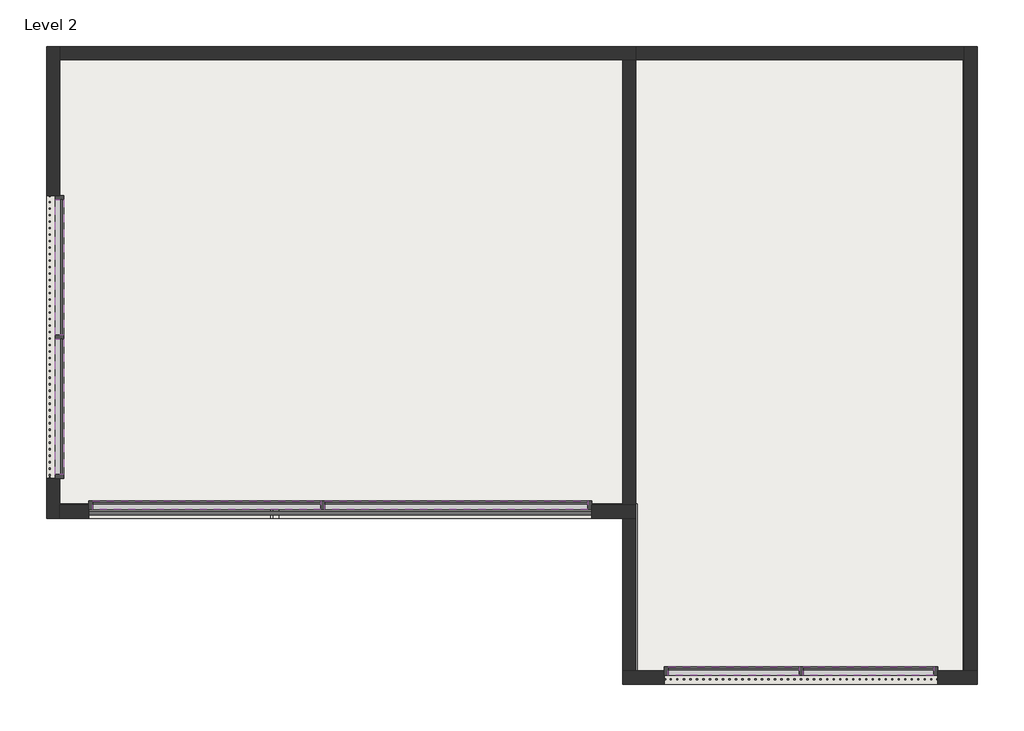
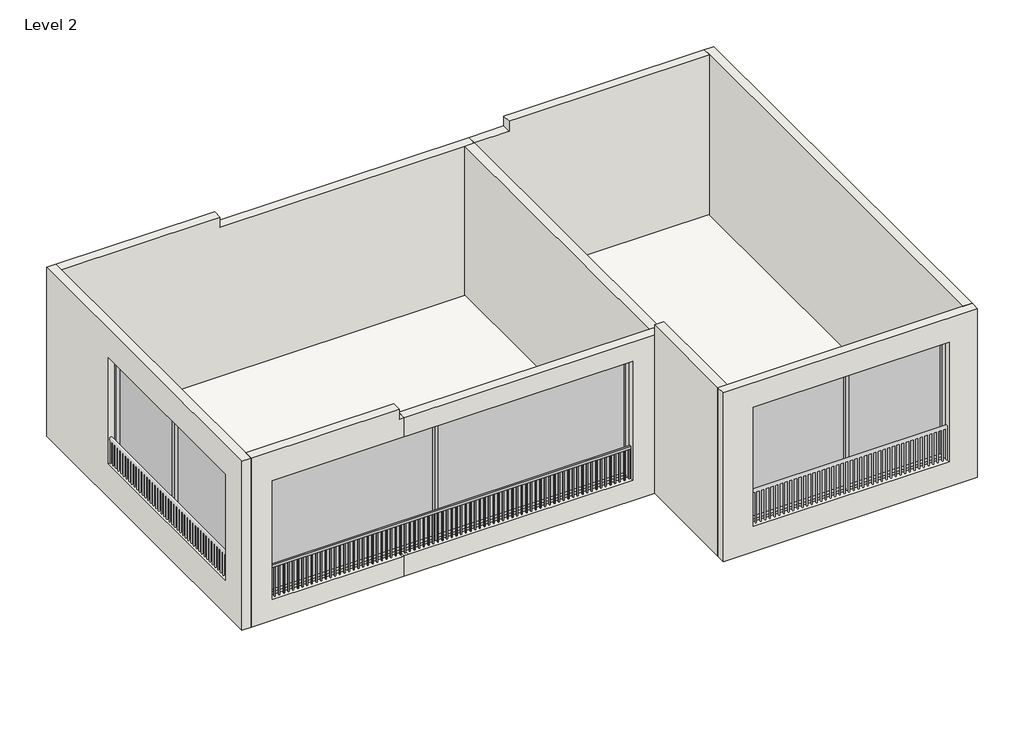
# One storey, part 1 of 2: 21 members, 9 walls, 6 plates, 1 railing, 1 roof.
"""IFC4 building model written with IfcOpenShell, lengths in millimetres."""

from ifc_helpers import new_model, si_unit, frame, origin, place, context, project, spatial, polyline, outline, extrude, faceted_brep, transform, mapped, element, save
from components import member_923d5781, member_d84c53df, member_a78380a5, member_2b402daf, member_c8ecc271, member_8f4b05ff, member_f0fea5a5, member_ee409385, system_panel_glazed_54db570c, system_panel_glazed_4346f86e, system_panel_glazed_ffba6474, system_panel_glazed_48ffcee9

model = new_model("IFC4")

# Units and contexts
model_context = context("Model", 3, world=origin())
ifc_project = project(units=[si_unit("LENGTHUNIT", "METRE", prefix="MILLI")], contexts=[model_context])

# Site, building, storey
site = spatial("IfcSite", under=ifc_project)
building = spatial("IfcBuilding", under=site)
storey = spatial("IfcBuildingStorey", under=building, Name="Level 2", Elevation=3657.6)

# Members
placement = place(None, origin())
member_shape = member_923d5781(model_context)
element("IfcMember", 1, ObjectType="Rectangular Mullion : 2.5\" x 5\" rectangular", at=placement, inside=storey, context=model_context, shape_type="MappedRepresentation", body=[
    mapped(member_shape, transform((-11752.6161748, -214.9874156, 4128.3774754), x_axis=(1.0, 0.0, 0.0), y_axis=(0.0, -1.0, 0.0), z_axis=(0.0, 0.0, -1.0))),
])
element("IfcMember", 2, ObjectType="Rectangular Mullion : 2.5\" x 5\" rectangular", at=placement, inside=storey, context=model_context, shape_type="MappedRepresentation", body=[
    mapped(member_shape, transform((-4288.9796605, -2805.7874156, 4241.0241774), x_axis=(1.0, 0.0, 0.0), y_axis=(0.0, -1.0, 0.0), z_axis=(0.0, 0.0, -1.0))),
])
member_2_shape = member_d84c53df(model_context)
element("IfcMember", 3, ObjectType="Rectangular Mullion : 2.5\" x 5\" rectangular", at=placement, inside=storey, context=model_context, shape_type="MappedRepresentation", body=[
    mapped(member_2_shape, transform((-7616.7372956, -214.9874156, 6871.5774754), x_axis=(0.0, 0.0, 1.0), y_axis=(0.0, -1.0, 0.0), z_axis=(1.0, 0.0, 0.0))),
])
element("IfcMember", 4, ObjectType="Rectangular Mullion : 2.5\" x 5\" rectangular", at=placement, inside=storey, context=model_context, shape_type="MappedRepresentation", body=[
    mapped(member_2_shape, transform((-11720.8661748, -214.9874156, 4128.3774754), x_axis=(0.0, 0.0, -1.0), y_axis=(0.0, -1.0, 0.0), z_axis=(-1.0, 0.0, 0.0))),
])
member_3_shape = member_a78380a5(model_context)
element("IfcMember", 5, ObjectType="Rectangular Mullion : 2.5\" x 5\" rectangular", at=placement, inside=storey, context=model_context, shape_type="MappedRepresentation", body=[
    mapped(member_3_shape, transform((-7553.2372956, -214.9874156, 4128.3774754), x_axis=(1.0, 0.0, 0.0), y_axis=(0.0, -1.0, 0.0), z_axis=(0.0, 0.0, -1.0))),
])
element("IfcMember", 6, ObjectType="Rectangular Mullion : 2.5\" x 5\" rectangular", at=placement, inside=storey, context=model_context, shape_type="MappedRepresentation", body=[
    mapped(member_3_shape, transform((-2155.3796605, -2805.7874156, 4241.0241774), x_axis=(1.0, 0.0, 0.0), y_axis=(0.0, -1.0, 0.0), z_axis=(0.0, 0.0, -1.0))),
])
member_4_shape = member_2b402daf(model_context)
element("IfcMember", 7, ObjectType="Rectangular Mullion : 2.5\" x 5\" rectangular", at=placement, inside=storey, context=model_context, shape_type="MappedRepresentation", body=[
    mapped(member_4_shape, transform((-11784.3661748, -214.9874156, 6871.5774754), x_axis=(0.0, 0.0, 1.0), y_axis=(0.0, -1.0, 0.0), z_axis=(1.0, 0.0, 0.0))),
])
element("IfcMember", 8, ObjectType="Rectangular Mullion : 2.5\" x 5\" rectangular", at=placement, inside=storey, context=model_context, shape_type="MappedRepresentation", body=[
    mapped(member_4_shape, transform((-15346.7161748, -214.9874156, 4128.3774754), x_axis=(0.0, 0.0, -1.0), y_axis=(0.0, -1.0, 0.0), z_axis=(-1.0, 0.0, 0.0))),
])
element("IfcMember", 9, ObjectType="Rectangular Mullion : 2.5\" x 5\" rectangular", at=placement, inside=storey, context=model_context, shape_type="MappedRepresentation", body=[
    mapped(member_3_shape, transform((-15410.2161748, -214.9874156, 6871.5774754), x_axis=(-1.0, 0.0, 0.0), y_axis=(0.0, -1.0, 0.0), z_axis=(0.0, 0.0, 1.0))),
])
element("IfcMember", 10, ObjectType="Rectangular Mullion : 2.5\" x 5\" rectangular", at=placement, inside=storey, context=model_context, shape_type="MappedRepresentation", body=[
    mapped(member_3_shape, transform((-6422.5796605, -2805.7874156, 6984.2241774), x_axis=(-1.0, 0.0, 0.0), y_axis=(0.0, -1.0, 0.0), z_axis=(0.0, 0.0, 1.0))),
])
member_5_shape = member_c8ecc271(model_context)
element("IfcMember", 11, ObjectType="Rectangular Mullion : 2.5\" x 5\" rectangular", at=placement, inside=storey, context=model_context, shape_type="MappedRepresentation", body=[
    mapped(member_5_shape, transform((-4320.7296605, -2805.7874156, 6984.2241774), x_axis=(0.0, 0.0, 1.0), y_axis=(0.0, -1.0, 0.0), z_axis=(1.0, 0.0, 0.0))),
])
element("IfcMember", 12, ObjectType="Rectangular Mullion : 2.5\" x 5\" rectangular", at=placement, inside=storey, context=model_context, shape_type="MappedRepresentation", body=[
    mapped(member_5_shape, transform((-2218.8796605, -2805.7874156, 6984.2241774), x_axis=(0.0, 0.0, 1.0), y_axis=(0.0, -1.0, 0.0), z_axis=(1.0, 0.0, 0.0))),
])
element("IfcMember", 13, ObjectType="Rectangular Mullion : 2.5\" x 5\" rectangular", at=placement, inside=storey, context=model_context, shape_type="MappedRepresentation", body=[
    mapped(member_5_shape, transform((-4257.2296605, -2805.7874156, 4241.0241774), x_axis=(0.0, 0.0, -1.0), y_axis=(0.0, -1.0, 0.0), z_axis=(-1.0, 0.0, 0.0))),
])
element("IfcMember", 14, ObjectType="Rectangular Mullion : 2.5\" x 5\" rectangular", at=placement, inside=storey, context=model_context, shape_type="MappedRepresentation", body=[
    mapped(member_5_shape, transform((-6359.0796605, -2805.7874156, 4241.0241774), x_axis=(0.0, 0.0, -1.0), y_axis=(0.0, -1.0, 0.0), z_axis=(-1.0, 0.0, 0.0))),
])
member_6_shape = member_8f4b05ff(model_context)
element("IfcMember", 15, ObjectType="Rectangular Mullion : 2.5\" x 5\" rectangular", at=placement, inside=storey, context=model_context, shape_type="MappedRepresentation", body=[
    mapped(member_6_shape, transform((-15861.8141623, 2443.1044753, 6871.5774754), x_axis=(0.0, 0.0, 1.0), y_axis=(-1.0, 0.0, 0.0), z_axis=(0.0, -1.0, 0.0))),
])
element("IfcMember", 16, ObjectType="Rectangular Mullion : 2.5\" x 5\" rectangular", at=placement, inside=storey, context=model_context, shape_type="MappedRepresentation", body=[
    mapped(member_6_shape, transform((-15861.8141623, 265.0544753, 6871.5774754), x_axis=(0.0, 0.0, 1.0), y_axis=(-1.0, 0.0, 0.0), z_axis=(0.0, -1.0, 0.0))),
])
member_7_shape = member_f0fea5a5(model_context)
element("IfcMember", 17, ObjectType="Rectangular Mullion : 2.5\" x 5\" rectangular", at=placement, inside=storey, context=model_context, shape_type="MappedRepresentation", body=[
    mapped(member_7_shape, transform((-15861.8141623, 2411.3544753, 4433.1774754), x_axis=(0.0, -1.0, 0.0), y_axis=(-1.0, 0.0, 0.0), z_axis=(0.0, 0.0, -1.0))),
])
element("IfcMember", 18, ObjectType="Rectangular Mullion : 2.5\" x 5\" rectangular", at=placement, inside=storey, context=model_context, shape_type="MappedRepresentation", body=[
    mapped(member_6_shape, transform((-15861.8141623, 2379.6044753, 4433.1774754), x_axis=(0.0, 0.0, -1.0), y_axis=(-1.0, 0.0, 0.0), z_axis=(0.0, 1.0, 0.0))),
])
element("IfcMember", 19, ObjectType="Rectangular Mullion : 2.5\" x 5\" rectangular", at=placement, inside=storey, context=model_context, shape_type="MappedRepresentation", body=[
    mapped(member_6_shape, transform((-15861.8141623, 4557.6544753, 4433.1774754), x_axis=(0.0, 0.0, -1.0), y_axis=(-1.0, 0.0, 0.0), z_axis=(0.0, 1.0, 0.0))),
])
member_8_shape = member_ee409385(model_context)
element("IfcMember", 20, ObjectType="Rectangular Mullion : 2.5\" x 5\" rectangular", at=placement, inside=storey, context=model_context, shape_type="MappedRepresentation", body=[
    mapped(member_8_shape, transform((-15861.8141623, 201.5544753, 4433.1774754), x_axis=(0.0, -1.0, 0.0), y_axis=(-1.0, 0.0, 0.0), z_axis=(0.0, 0.0, -1.0))),
])
element("IfcMember", 21, ObjectType="Rectangular Mullion : 2.5\" x 5\" rectangular", at=placement, inside=storey, context=model_context, shape_type="MappedRepresentation", body=[
    mapped(member_8_shape, transform((-15861.8141623, 4621.1544753, 6871.5774754), x_axis=(0.0, 1.0, 0.0), y_axis=(-1.0, 0.0, 0.0), z_axis=(0.0, 0.0, 1.0))),
])

# Plates
system_panel_glazed_shape = system_panel_glazed_54db570c(model_context)
element("IfcPlate", 22, ObjectType="System Panel : Glazed", at=placement, inside=storey, context=model_context, shape_type="MappedRepresentation", body=[
    mapped(system_panel_glazed_shape, transform((-9668.8017352, -214.9874156, 4191.8774754), x_axis=(1.0, 0.0, 0.0), y_axis=(0.0, 1.0, 0.0), z_axis=(0.0, 0.0, 1.0))),
])
system_panel_glazed_2_shape = system_panel_glazed_4346f86e(model_context)
element("IfcPlate", 23, ObjectType="System Panel : Glazed", at=placement, inside=storey, context=model_context, shape_type="MappedRepresentation", body=[
    mapped(system_panel_glazed_2_shape, transform((-13565.5411748, -214.9874156, 4191.8774754), x_axis=(1.0, 0.0, 0.0), y_axis=(0.0, 1.0, 0.0), z_axis=(0.0, 0.0, 1.0))),
])
system_panel_glazed_3_shape = system_panel_glazed_ffba6474(model_context)
element("IfcPlate", 24, ObjectType="System Panel : Glazed", at=placement, inside=storey, context=model_context, shape_type="MappedRepresentation", body=[
    mapped(system_panel_glazed_3_shape, transform((-5339.9046605, -2805.7874156, 4304.5241774), x_axis=(1.0, 0.0, 0.0), y_axis=(0.0, 1.0, 0.0), z_axis=(0.0, 0.0, 1.0))),
])
element("IfcPlate", 25, ObjectType="System Panel : Glazed", at=placement, inside=storey, context=model_context, shape_type="MappedRepresentation", body=[
    mapped(system_panel_glazed_3_shape, transform((-3238.0546605, -2805.7874156, 4304.5241774), x_axis=(1.0, 0.0, 0.0), y_axis=(0.0, 1.0, 0.0), z_axis=(0.0, 0.0, 1.0))),
])
system_panel_glazed_4_shape = system_panel_glazed_48ffcee9(model_context)
element("IfcPlate", 26, ObjectType="System Panel : Glazed", at=placement, inside=storey, context=model_context, shape_type="MappedRepresentation", body=[
    mapped(system_panel_glazed_4_shape, transform((-15861.8141623, 3500.3794753, 4496.6774754), x_axis=(0.0, -1.0, 0.0), y_axis=(1.0, 0.0, 0.0), z_axis=(0.0, 0.0, 1.0))),
])
element("IfcPlate", 27, ObjectType="System Panel : Glazed", at=placement, inside=storey, context=model_context, shape_type="MappedRepresentation", body=[
    mapped(system_panel_glazed_4_shape, transform((-15861.8141623, 1322.3294753, 4496.6774754), x_axis=(0.0, -1.0, 0.0), y_axis=(1.0, 0.0, 0.0), z_axis=(0.0, 0.0, 1.0))),
])

# Railing
element("IfcRailing", 28, ObjectType="Handrail - Rectangular", at=placement, inside=storey, context=model_context, shape_type="SweptSolid", body=[
    extrude(outline(polyline([(-15410.2161748, -367.3874156), (-15410.2161748, -316.5874156), (-7553.2372956, -316.5874156), (-7553.2372956, -367.3874156), (-15410.2161748, -367.3874156)])), frame((0.0, 0.0, 4826.0), z_axis=(0.0, 0.0, 1.0), x_axis=(1.0, 0.0, 0.0)), (0.0, 0.0, 1.0), 50.8),
    extrude(outline(polyline([(-7596.5411748, -351.5124156), (-7596.5411748, -332.4624156), (-7577.4911748, -332.4624156), (-7577.4911748, -351.5124156), (-7596.5411748, -351.5124156)])), frame((0.0, 0.0, 3962.4), z_axis=(0.0, 0.0, 1.0), x_axis=(1.0, 0.0, 0.0)), (0.0, 0.0, 1.0), 863.6),
    extrude(outline(polyline([(-7698.1411748, -351.5124156), (-7698.1411748, -332.4624156), (-7679.0911748, -332.4624156), (-7679.0911748, -351.5124156), (-7698.1411748, -351.5124156)])), frame((0.0, 0.0, 3962.4), z_axis=(0.0, 0.0, 1.0), x_axis=(1.0, 0.0, 0.0)), (0.0, 0.0, 1.0), 863.6),
    extrude(outline(polyline([(-7799.7411748, -351.5124156), (-7799.7411748, -332.4624156), (-7780.6911748, -332.4624156), (-7780.6911748, -351.5124156), (-7799.7411748, -351.5124156)])), frame((0.0, 0.0, 3962.4), z_axis=(0.0, 0.0, 1.0), x_axis=(1.0, 0.0, 0.0)), (0.0, 0.0, 1.0), 863.6),
    extrude(outline(polyline([(-7901.3411748, -351.5124156), (-7901.3411748, -332.4624156), (-7882.2911748, -332.4624156), (-7882.2911748, -351.5124156), (-7901.3411748, -351.5124156)])), frame((0.0, 0.0, 3962.4), z_axis=(0.0, 0.0, 1.0), x_axis=(1.0, 0.0, 0.0)), (0.0, 0.0, 1.0), 863.6),
    extrude(outline(polyline([(-8002.9411748, -351.5124156), (-8002.9411748, -332.4624156), (-7983.8911748, -332.4624156), (-7983.8911748, -351.5124156), (-8002.9411748, -351.5124156)])), frame((0.0, 0.0, 3962.4), z_axis=(0.0, 0.0, 1.0), x_axis=(1.0, 0.0, 0.0)), (0.0, 0.0, 1.0), 863.6),
    extrude(outline(polyline([(-8104.5411748, -351.5124156), (-8104.5411748, -332.4624156), (-8085.4911748, -332.4624156), (-8085.4911748, -351.5124156), (-8104.5411748, -351.5124156)])), frame((0.0, 0.0, 3962.4), z_axis=(0.0, 0.0, 1.0), x_axis=(1.0, 0.0, 0.0)), (0.0, 0.0, 1.0), 863.6),
    extrude(outline(polyline([(-8206.1411748, -351.5124156), (-8206.1411748, -332.4624156), (-8187.0911748, -332.4624156), (-8187.0911748, -351.5124156), (-8206.1411748, -351.5124156)])), frame((0.0, 0.0, 3962.4), z_axis=(0.0, 0.0, 1.0), x_axis=(1.0, 0.0, 0.0)), (0.0, 0.0, 1.0), 863.6),
    extrude(outline(polyline([(-8307.7411748, -351.5124156), (-8307.7411748, -332.4624156), (-8288.6911748, -332.4624156), (-8288.6911748, -351.5124156), (-8307.7411748, -351.5124156)])), frame((0.0, 0.0, 3962.4), z_axis=(0.0, 0.0, 1.0), x_axis=(1.0, 0.0, 0.0)), (0.0, 0.0, 1.0), 863.6),
    extrude(outline(polyline([(-8409.3411748, -351.5124156), (-8409.3411748, -332.4624156), (-8390.2911748, -332.4624156), (-8390.2911748, -351.5124156), (-8409.3411748, -351.5124156)])), frame((0.0, 0.0, 3962.4), z_axis=(0.0, 0.0, 1.0), x_axis=(1.0, 0.0, 0.0)), (0.0, 0.0, 1.0), 863.6),
    extrude(outline(polyline([(-8510.9411748, -351.5124156), (-8510.9411748, -332.4624156), (-8491.8911748, -332.4624156), (-8491.8911748, -351.5124156), (-8510.9411748, -351.5124156)])), frame((0.0, 0.0, 3962.4), z_axis=(0.0, 0.0, 1.0), x_axis=(1.0, 0.0, 0.0)), (0.0, 0.0, 1.0), 863.6),
    extrude(outline(polyline([(-8612.5411748, -351.5124156), (-8612.5411748, -332.4624156), (-8593.4911748, -332.4624156), (-8593.4911748, -351.5124156), (-8612.5411748, -351.5124156)])), frame((0.0, 0.0, 3962.4), z_axis=(0.0, 0.0, 1.0), x_axis=(1.0, 0.0, 0.0)), (0.0, 0.0, 1.0), 863.6),
    extrude(outline(polyline([(-8714.1411748, -351.5124156), (-8714.1411748, -332.4624156), (-8695.0911748, -332.4624156), (-8695.0911748, -351.5124156), (-8714.1411748, -351.5124156)])), frame((0.0, 0.0, 3962.4), z_axis=(0.0, 0.0, 1.0), x_axis=(1.0, 0.0, 0.0)), (0.0, 0.0, 1.0), 863.6),
    extrude(outline(polyline([(-8815.7411748, -351.5124156), (-8815.7411748, -332.4624156), (-8796.6911748, -332.4624156), (-8796.6911748, -351.5124156), (-8815.7411748, -351.5124156)])), frame((0.0, 0.0, 3962.4), z_axis=(0.0, 0.0, 1.0), x_axis=(1.0, 0.0, 0.0)), (0.0, 0.0, 1.0), 863.6),
    extrude(outline(polyline([(-8917.3411748, -351.5124156), (-8917.3411748, -332.4624156), (-8898.2911748, -332.4624156), (-8898.2911748, -351.5124156), (-8917.3411748, -351.5124156)])), frame((0.0, 0.0, 3962.4), z_axis=(0.0, 0.0, 1.0), x_axis=(1.0, 0.0, 0.0)), (0.0, 0.0, 1.0), 863.6),
    extrude(outline(polyline([(-9018.9411748, -351.5124156), (-9018.9411748, -332.4624156), (-8999.8911748, -332.4624156), (-8999.8911748, -351.5124156), (-9018.9411748, -351.5124156)])), frame((0.0, 0.0, 3962.4), z_axis=(0.0, 0.0, 1.0), x_axis=(1.0, 0.0, 0.0)), (0.0, 0.0, 1.0), 863.6),
    extrude(outline(polyline([(-9120.5411748, -351.5124156), (-9120.5411748, -332.4624156), (-9101.4911748, -332.4624156), (-9101.4911748, -351.5124156), (-9120.5411748, -351.5124156)])), frame((0.0, 0.0, 3962.4), z_axis=(0.0, 0.0, 1.0), x_axis=(1.0, 0.0, 0.0)), (0.0, 0.0, 1.0), 863.6),
    extrude(outline(polyline([(-9222.1411748, -351.5124156), (-9222.1411748, -332.4624156), (-9203.0911748, -332.4624156), (-9203.0911748, -351.5124156), (-9222.1411748, -351.5124156)])), frame((0.0, 0.0, 3962.4), z_axis=(0.0, 0.0, 1.0), x_axis=(1.0, 0.0, 0.0)), (0.0, 0.0, 1.0), 863.6),
    extrude(outline(polyline([(-9323.7411748, -351.5124156), (-9323.7411748, -332.4624156), (-9304.6911748, -332.4624156), (-9304.6911748, -351.5124156), (-9323.7411748, -351.5124156)])), frame((0.0, 0.0, 3962.4), z_axis=(0.0, 0.0, 1.0), x_axis=(1.0, 0.0, 0.0)), (0.0, 0.0, 1.0), 863.6),
    extrude(outline(polyline([(-9425.3411748, -351.5124156), (-9425.3411748, -332.4624156), (-9406.2911748, -332.4624156), (-9406.2911748, -351.5124156), (-9425.3411748, -351.5124156)])), frame((0.0, 0.0, 3962.4), z_axis=(0.0, 0.0, 1.0), x_axis=(1.0, 0.0, 0.0)), (0.0, 0.0, 1.0), 863.6),
    extrude(outline(polyline([(-9526.9411748, -351.5124156), (-9526.9411748, -332.4624156), (-9507.8911748, -332.4624156), (-9507.8911748, -351.5124156), (-9526.9411748, -351.5124156)])), frame((0.0, 0.0, 3962.4), z_axis=(0.0, 0.0, 1.0), x_axis=(1.0, 0.0, 0.0)), (0.0, 0.0, 1.0), 863.6),
    extrude(outline(polyline([(-9628.5411748, -351.5124156), (-9628.5411748, -332.4624156), (-9609.4911748, -332.4624156), (-9609.4911748, -351.5124156), (-9628.5411748, -351.5124156)])), frame((0.0, 0.0, 3962.4), z_axis=(0.0, 0.0, 1.0), x_axis=(1.0, 0.0, 0.0)), (0.0, 0.0, 1.0), 863.6),
    extrude(outline(polyline([(-9730.1411748, -351.5124156), (-9730.1411748, -332.4624156), (-9711.0911748, -332.4624156), (-9711.0911748, -351.5124156), (-9730.1411748, -351.5124156)])), frame((0.0, 0.0, 3962.4), z_axis=(0.0, 0.0, 1.0), x_axis=(1.0, 0.0, 0.0)), (0.0, 0.0, 1.0), 863.6),
    extrude(outline(polyline([(-9831.7411748, -351.5124156), (-9831.7411748, -332.4624156), (-9812.6911748, -332.4624156), (-9812.6911748, -351.5124156), (-9831.7411748, -351.5124156)])), frame((0.0, 0.0, 3962.4), z_axis=(0.0, 0.0, 1.0), x_axis=(1.0, 0.0, 0.0)), (0.0, 0.0, 1.0), 863.6),
    extrude(outline(polyline([(-9933.3411748, -351.5124156), (-9933.3411748, -332.4624156), (-9914.2911748, -332.4624156), (-9914.2911748, -351.5124156), (-9933.3411748, -351.5124156)])), frame((0.0, 0.0, 3962.4), z_axis=(0.0, 0.0, 1.0), x_axis=(1.0, 0.0, 0.0)), (0.0, 0.0, 1.0), 863.6),
    extrude(outline(polyline([(-10034.9411748, -351.5124156), (-10034.9411748, -332.4624156), (-10015.8911748, -332.4624156), (-10015.8911748, -351.5124156), (-10034.9411748, -351.5124156)])), frame((0.0, 0.0, 3962.4), z_axis=(0.0, 0.0, 1.0), x_axis=(1.0, 0.0, 0.0)), (0.0, 0.0, 1.0), 863.6),
    extrude(outline(polyline([(-10136.5411748, -351.5124156), (-10136.5411748, -332.4624156), (-10117.4911748, -332.4624156), (-10117.4911748, -351.5124156), (-10136.5411748, -351.5124156)])), frame((0.0, 0.0, 3962.4), z_axis=(0.0, 0.0, 1.0), x_axis=(1.0, 0.0, 0.0)), (0.0, 0.0, 1.0), 863.6),
    extrude(outline(polyline([(-10238.1411748, -351.5124156), (-10238.1411748, -332.4624156), (-10219.0911748, -332.4624156), (-10219.0911748, -351.5124156), (-10238.1411748, -351.5124156)])), frame((0.0, 0.0, 3962.4), z_axis=(0.0, 0.0, 1.0), x_axis=(1.0, 0.0, 0.0)), (0.0, 0.0, 1.0), 863.6),
    extrude(outline(polyline([(-10339.7411748, -351.5124156), (-10339.7411748, -332.4624156), (-10320.6911748, -332.4624156), (-10320.6911748, -351.5124156), (-10339.7411748, -351.5124156)])), frame((0.0, 0.0, 3962.4), z_axis=(0.0, 0.0, 1.0), x_axis=(1.0, 0.0, 0.0)), (0.0, 0.0, 1.0), 863.6),
    extrude(outline(polyline([(-10441.3411748, -351.5124156), (-10441.3411748, -332.4624156), (-10422.2911748, -332.4624156), (-10422.2911748, -351.5124156), (-10441.3411748, -351.5124156)])), frame((0.0, 0.0, 3962.4), z_axis=(0.0, 0.0, 1.0), x_axis=(1.0, 0.0, 0.0)), (0.0, 0.0, 1.0), 863.6),
    extrude(outline(polyline([(-10542.9411748, -351.5124156), (-10542.9411748, -332.4624156), (-10523.8911748, -332.4624156), (-10523.8911748, -351.5124156), (-10542.9411748, -351.5124156)])), frame((0.0, 0.0, 3962.4), z_axis=(0.0, 0.0, 1.0), x_axis=(1.0, 0.0, 0.0)), (0.0, 0.0, 1.0), 863.6),
    extrude(outline(polyline([(-10644.5411748, -351.5124156), (-10644.5411748, -332.4624156), (-10625.4911748, -332.4624156), (-10625.4911748, -351.5124156), (-10644.5411748, -351.5124156)])), frame((0.0, 0.0, 3962.4), z_axis=(0.0, 0.0, 1.0), x_axis=(1.0, 0.0, 0.0)), (0.0, 0.0, 1.0), 863.6),
    extrude(outline(polyline([(-10746.1411748, -351.5124156), (-10746.1411748, -332.4624156), (-10727.0911748, -332.4624156), (-10727.0911748, -351.5124156), (-10746.1411748, -351.5124156)])), frame((0.0, 0.0, 3962.4), z_axis=(0.0, 0.0, 1.0), x_axis=(1.0, 0.0, 0.0)), (0.0, 0.0, 1.0), 863.6),
    extrude(outline(polyline([(-10847.7411748, -351.5124156), (-10847.7411748, -332.4624156), (-10828.6911748, -332.4624156), (-10828.6911748, -351.5124156), (-10847.7411748, -351.5124156)])), frame((0.0, 0.0, 3962.4), z_axis=(0.0, 0.0, 1.0), x_axis=(1.0, 0.0, 0.0)), (0.0, 0.0, 1.0), 863.6),
    extrude(outline(polyline([(-10949.3411748, -351.5124156), (-10949.3411748, -332.4624156), (-10930.2911748, -332.4624156), (-10930.2911748, -351.5124156), (-10949.3411748, -351.5124156)])), frame((0.0, 0.0, 3962.4), z_axis=(0.0, 0.0, 1.0), x_axis=(1.0, 0.0, 0.0)), (0.0, 0.0, 1.0), 863.6),
    extrude(outline(polyline([(-11050.9411748, -351.5124156), (-11050.9411748, -332.4624156), (-11031.8911748, -332.4624156), (-11031.8911748, -351.5124156), (-11050.9411748, -351.5124156)])), frame((0.0, 0.0, 3962.4), z_axis=(0.0, 0.0, 1.0), x_axis=(1.0, 0.0, 0.0)), (0.0, 0.0, 1.0), 863.6),
    extrude(outline(polyline([(-11152.5411748, -351.5124156), (-11152.5411748, -332.4624156), (-11133.4911748, -332.4624156), (-11133.4911748, -351.5124156), (-11152.5411748, -351.5124156)])), frame((0.0, 0.0, 3962.4), z_axis=(0.0, 0.0, 1.0), x_axis=(1.0, 0.0, 0.0)), (0.0, 0.0, 1.0), 863.6),
    extrude(outline(polyline([(-11254.1411748, -351.5124156), (-11254.1411748, -332.4624156), (-11235.0911748, -332.4624156), (-11235.0911748, -351.5124156), (-11254.1411748, -351.5124156)])), frame((0.0, 0.0, 3962.4), z_axis=(0.0, 0.0, 1.0), x_axis=(1.0, 0.0, 0.0)), (0.0, 0.0, 1.0), 863.6),
    extrude(outline(polyline([(-11355.7411748, -351.5124156), (-11355.7411748, -332.4624156), (-11336.6911748, -332.4624156), (-11336.6911748, -351.5124156), (-11355.7411748, -351.5124156)])), frame((0.0, 0.0, 3962.4), z_axis=(0.0, 0.0, 1.0), x_axis=(1.0, 0.0, 0.0)), (0.0, 0.0, 1.0), 863.6),
    extrude(outline(polyline([(-11457.3411748, -351.5124156), (-11457.3411748, -332.4624156), (-11438.2911748, -332.4624156), (-11438.2911748, -351.5124156), (-11457.3411748, -351.5124156)])), frame((0.0, 0.0, 3962.4), z_axis=(0.0, 0.0, 1.0), x_axis=(1.0, 0.0, 0.0)), (0.0, 0.0, 1.0), 863.6),
    extrude(outline(polyline([(-11558.9411748, -351.5124156), (-11558.9411748, -332.4624156), (-11539.8911748, -332.4624156), (-11539.8911748, -351.5124156), (-11558.9411748, -351.5124156)])), frame((0.0, 0.0, 3962.4), z_axis=(0.0, 0.0, 1.0), x_axis=(1.0, 0.0, 0.0)), (0.0, 0.0, 1.0), 863.6),
    extrude(outline(polyline([(-11660.5411748, -351.5124156), (-11660.5411748, -332.4624156), (-11641.4911748, -332.4624156), (-11641.4911748, -351.5124156), (-11660.5411748, -351.5124156)])), frame((0.0, 0.0, 3962.4), z_axis=(0.0, 0.0, 1.0), x_axis=(1.0, 0.0, 0.0)), (0.0, 0.0, 1.0), 863.6),
    extrude(outline(polyline([(-11762.1411748, -351.5124156), (-11762.1411748, -332.4624156), (-11743.0911748, -332.4624156), (-11743.0911748, -351.5124156), (-11762.1411748, -351.5124156)])), frame((0.0, 0.0, 3962.4), z_axis=(0.0, 0.0, 1.0), x_axis=(1.0, 0.0, 0.0)), (0.0, 0.0, 1.0), 863.6),
    extrude(outline(polyline([(-11863.7411748, -351.5124156), (-11863.7411748, -332.4624156), (-11844.6911748, -332.4624156), (-11844.6911748, -351.5124156), (-11863.7411748, -351.5124156)])), frame((0.0, 0.0, 3962.4), z_axis=(0.0, 0.0, 1.0), x_axis=(1.0, 0.0, 0.0)), (0.0, 0.0, 1.0), 863.6),
    extrude(outline(polyline([(-11965.3411748, -351.5124156), (-11965.3411748, -332.4624156), (-11946.2911748, -332.4624156), (-11946.2911748, -351.5124156), (-11965.3411748, -351.5124156)])), frame((0.0, 0.0, 3962.4), z_axis=(0.0, 0.0, 1.0), x_axis=(1.0, 0.0, 0.0)), (0.0, 0.0, 1.0), 863.6),
    extrude(outline(polyline([(-12066.9411748, -351.5124156), (-12066.9411748, -332.4624156), (-12047.8911748, -332.4624156), (-12047.8911748, -351.5124156), (-12066.9411748, -351.5124156)])), frame((0.0, 0.0, 3962.4), z_axis=(0.0, 0.0, 1.0), x_axis=(1.0, 0.0, 0.0)), (0.0, 0.0, 1.0), 863.6),
    extrude(outline(polyline([(-12168.5411748, -351.5124156), (-12168.5411748, -332.4624156), (-12149.4911748, -332.4624156), (-12149.4911748, -351.5124156), (-12168.5411748, -351.5124156)])), frame((0.0, 0.0, 3962.4), z_axis=(0.0, 0.0, 1.0), x_axis=(1.0, 0.0, 0.0)), (0.0, 0.0, 1.0), 863.6),
    extrude(outline(polyline([(-12270.1411748, -351.5124156), (-12270.1411748, -332.4624156), (-12251.0911748, -332.4624156), (-12251.0911748, -351.5124156), (-12270.1411748, -351.5124156)])), frame((0.0, 0.0, 3962.4), z_axis=(0.0, 0.0, 1.0), x_axis=(1.0, 0.0, 0.0)), (0.0, 0.0, 1.0), 863.6),
    extrude(outline(polyline([(-12371.7411748, -351.5124156), (-12371.7411748, -332.4624156), (-12352.6911748, -332.4624156), (-12352.6911748, -351.5124156), (-12371.7411748, -351.5124156)])), frame((0.0, 0.0, 3962.4), z_axis=(0.0, 0.0, 1.0), x_axis=(1.0, 0.0, 0.0)), (0.0, 0.0, 1.0), 863.6),
    extrude(outline(polyline([(-12473.3411748, -351.5124156), (-12473.3411748, -332.4624156), (-12454.2911748, -332.4624156), (-12454.2911748, -351.5124156), (-12473.3411748, -351.5124156)])), frame((0.0, 0.0, 3962.4), z_axis=(0.0, 0.0, 1.0), x_axis=(1.0, 0.0, 0.0)), (0.0, 0.0, 1.0), 863.6),
    extrude(outline(polyline([(-12574.9411748, -351.5124156), (-12574.9411748, -332.4624156), (-12555.8911748, -332.4624156), (-12555.8911748, -351.5124156), (-12574.9411748, -351.5124156)])), frame((0.0, 0.0, 3962.4), z_axis=(0.0, 0.0, 1.0), x_axis=(1.0, 0.0, 0.0)), (0.0, 0.0, 1.0), 863.6),
    extrude(outline(polyline([(-12676.5411748, -351.5124156), (-12676.5411748, -332.4624156), (-12657.4911748, -332.4624156), (-12657.4911748, -351.5124156), (-12676.5411748, -351.5124156)])), frame((0.0, 0.0, 3962.4), z_axis=(0.0, 0.0, 1.0), x_axis=(1.0, 0.0, 0.0)), (0.0, 0.0, 1.0), 863.6),
    extrude(outline(polyline([(-12778.1411748, -351.5124156), (-12778.1411748, -332.4624156), (-12759.0911748, -332.4624156), (-12759.0911748, -351.5124156), (-12778.1411748, -351.5124156)])), frame((0.0, 0.0, 3962.4), z_axis=(0.0, 0.0, 1.0), x_axis=(1.0, 0.0, 0.0)), (0.0, 0.0, 1.0), 863.6),
    extrude(outline(polyline([(-12879.7411748, -351.5124156), (-12879.7411748, -332.4624156), (-12860.6911748, -332.4624156), (-12860.6911748, -351.5124156), (-12879.7411748, -351.5124156)])), frame((0.0, 0.0, 3962.4), z_axis=(0.0, 0.0, 1.0), x_axis=(1.0, 0.0, 0.0)), (0.0, 0.0, 1.0), 863.6),
    extrude(outline(polyline([(-12981.3411748, -351.5124156), (-12981.3411748, -332.4624156), (-12962.2911748, -332.4624156), (-12962.2911748, -351.5124156), (-12981.3411748, -351.5124156)])), frame((0.0, 0.0, 3962.4), z_axis=(0.0, 0.0, 1.0), x_axis=(1.0, 0.0, 0.0)), (0.0, 0.0, 1.0), 863.6),
    extrude(outline(polyline([(-13082.9411748, -351.5124156), (-13082.9411748, -332.4624156), (-13063.8911748, -332.4624156), (-13063.8911748, -351.5124156), (-13082.9411748, -351.5124156)])), frame((0.0, 0.0, 3962.4), z_axis=(0.0, 0.0, 1.0), x_axis=(1.0, 0.0, 0.0)), (0.0, 0.0, 1.0), 863.6),
    extrude(outline(polyline([(-13184.5411748, -351.5124156), (-13184.5411748, -332.4624156), (-13165.4911748, -332.4624156), (-13165.4911748, -351.5124156), (-13184.5411748, -351.5124156)])), frame((0.0, 0.0, 3962.4), z_axis=(0.0, 0.0, 1.0), x_axis=(1.0, 0.0, 0.0)), (0.0, 0.0, 1.0), 863.6),
    extrude(outline(polyline([(-13286.1411748, -351.5124156), (-13286.1411748, -332.4624156), (-13267.0911748, -332.4624156), (-13267.0911748, -351.5124156), (-13286.1411748, -351.5124156)])), frame((0.0, 0.0, 3962.4), z_axis=(0.0, 0.0, 1.0), x_axis=(1.0, 0.0, 0.0)), (0.0, 0.0, 1.0), 863.6),
    extrude(outline(polyline([(-13387.7411748, -351.5124156), (-13387.7411748, -332.4624156), (-13368.6911748, -332.4624156), (-13368.6911748, -351.5124156), (-13387.7411748, -351.5124156)])), frame((0.0, 0.0, 3962.4), z_axis=(0.0, 0.0, 1.0), x_axis=(1.0, 0.0, 0.0)), (0.0, 0.0, 1.0), 863.6),
    extrude(outline(polyline([(-13489.3411748, -351.5124156), (-13489.3411748, -332.4624156), (-13470.2911748, -332.4624156), (-13470.2911748, -351.5124156), (-13489.3411748, -351.5124156)])), frame((0.0, 0.0, 3962.4), z_axis=(0.0, 0.0, 1.0), x_axis=(1.0, 0.0, 0.0)), (0.0, 0.0, 1.0), 863.6),
    extrude(outline(polyline([(-13590.9411748, -351.5124156), (-13590.9411748, -332.4624156), (-13571.8911748, -332.4624156), (-13571.8911748, -351.5124156), (-13590.9411748, -351.5124156)])), frame((0.0, 0.0, 3962.4), z_axis=(0.0, 0.0, 1.0), x_axis=(1.0, 0.0, 0.0)), (0.0, 0.0, 1.0), 863.6),
    extrude(outline(polyline([(-13692.5411748, -351.5124156), (-13692.5411748, -332.4624156), (-13673.4911748, -332.4624156), (-13673.4911748, -351.5124156), (-13692.5411748, -351.5124156)])), frame((0.0, 0.0, 3962.4), z_axis=(0.0, 0.0, 1.0), x_axis=(1.0, 0.0, 0.0)), (0.0, 0.0, 1.0), 863.6),
    extrude(outline(polyline([(-13794.1411748, -351.5124156), (-13794.1411748, -332.4624156), (-13775.0911748, -332.4624156), (-13775.0911748, -351.5124156), (-13794.1411748, -351.5124156)])), frame((0.0, 0.0, 3962.4), z_axis=(0.0, 0.0, 1.0), x_axis=(1.0, 0.0, 0.0)), (0.0, 0.0, 1.0), 863.6),
    extrude(outline(polyline([(-13895.7411748, -351.5124156), (-13895.7411748, -332.4624156), (-13876.6911748, -332.4624156), (-13876.6911748, -351.5124156), (-13895.7411748, -351.5124156)])), frame((0.0, 0.0, 3962.4), z_axis=(0.0, 0.0, 1.0), x_axis=(1.0, 0.0, 0.0)), (0.0, 0.0, 1.0), 863.6),
    extrude(outline(polyline([(-13997.3411748, -351.5124156), (-13997.3411748, -332.4624156), (-13978.2911748, -332.4624156), (-13978.2911748, -351.5124156), (-13997.3411748, -351.5124156)])), frame((0.0, 0.0, 3962.4), z_axis=(0.0, 0.0, 1.0), x_axis=(1.0, 0.0, 0.0)), (0.0, 0.0, 1.0), 863.6),
    extrude(outline(polyline([(-14098.9411748, -351.5124156), (-14098.9411748, -332.4624156), (-14079.8911748, -332.4624156), (-14079.8911748, -351.5124156), (-14098.9411748, -351.5124156)])), frame((0.0, 0.0, 3962.4), z_axis=(0.0, 0.0, 1.0), x_axis=(1.0, 0.0, 0.0)), (0.0, 0.0, 1.0), 863.6),
    extrude(outline(polyline([(-14200.5411748, -351.5124156), (-14200.5411748, -332.4624156), (-14181.4911748, -332.4624156), (-14181.4911748, -351.5124156), (-14200.5411748, -351.5124156)])), frame((0.0, 0.0, 3962.4), z_axis=(0.0, 0.0, 1.0), x_axis=(1.0, 0.0, 0.0)), (0.0, 0.0, 1.0), 863.6),
    extrude(outline(polyline([(-14302.1411748, -351.5124156), (-14302.1411748, -332.4624156), (-14283.0911748, -332.4624156), (-14283.0911748, -351.5124156), (-14302.1411748, -351.5124156)])), frame((0.0, 0.0, 3962.4), z_axis=(0.0, 0.0, 1.0), x_axis=(1.0, 0.0, 0.0)), (0.0, 0.0, 1.0), 863.6),
    extrude(outline(polyline([(-14403.7411748, -351.5124156), (-14403.7411748, -332.4624156), (-14384.6911748, -332.4624156), (-14384.6911748, -351.5124156), (-14403.7411748, -351.5124156)])), frame((0.0, 0.0, 3962.4), z_axis=(0.0, 0.0, 1.0), x_axis=(1.0, 0.0, 0.0)), (0.0, 0.0, 1.0), 863.6),
    extrude(outline(polyline([(-14505.3411748, -351.5124156), (-14505.3411748, -332.4624156), (-14486.2911748, -332.4624156), (-14486.2911748, -351.5124156), (-14505.3411748, -351.5124156)])), frame((0.0, 0.0, 3962.4), z_axis=(0.0, 0.0, 1.0), x_axis=(1.0, 0.0, 0.0)), (0.0, 0.0, 1.0), 863.6),
    extrude(outline(polyline([(-14606.9411748, -351.5124156), (-14606.9411748, -332.4624156), (-14587.8911748, -332.4624156), (-14587.8911748, -351.5124156), (-14606.9411748, -351.5124156)])), frame((0.0, 0.0, 3962.4), z_axis=(0.0, 0.0, 1.0), x_axis=(1.0, 0.0, 0.0)), (0.0, 0.0, 1.0), 863.6),
    extrude(outline(polyline([(-14708.5411748, -351.5124156), (-14708.5411748, -332.4624156), (-14689.4911748, -332.4624156), (-14689.4911748, -351.5124156), (-14708.5411748, -351.5124156)])), frame((0.0, 0.0, 3962.4), z_axis=(0.0, 0.0, 1.0), x_axis=(1.0, 0.0, 0.0)), (0.0, 0.0, 1.0), 863.6),
    extrude(outline(polyline([(-14810.1411748, -351.5124156), (-14810.1411748, -332.4624156), (-14791.0911748, -332.4624156), (-14791.0911748, -351.5124156), (-14810.1411748, -351.5124156)])), frame((0.0, 0.0, 3962.4), z_axis=(0.0, 0.0, 1.0), x_axis=(1.0, 0.0, 0.0)), (0.0, 0.0, 1.0), 863.6),
    extrude(outline(polyline([(-14911.7411748, -351.5124156), (-14911.7411748, -332.4624156), (-14892.6911748, -332.4624156), (-14892.6911748, -351.5124156), (-14911.7411748, -351.5124156)])), frame((0.0, 0.0, 3962.4), z_axis=(0.0, 0.0, 1.0), x_axis=(1.0, 0.0, 0.0)), (0.0, 0.0, 1.0), 863.6),
    extrude(outline(polyline([(-15013.3411748, -351.5124156), (-15013.3411748, -332.4624156), (-14994.2911748, -332.4624156), (-14994.2911748, -351.5124156), (-15013.3411748, -351.5124156)])), frame((0.0, 0.0, 3962.4), z_axis=(0.0, 0.0, 1.0), x_axis=(1.0, 0.0, 0.0)), (0.0, 0.0, 1.0), 863.6),
    extrude(outline(polyline([(-15114.9411748, -351.5124156), (-15114.9411748, -332.4624156), (-15095.8911748, -332.4624156), (-15095.8911748, -351.5124156), (-15114.9411748, -351.5124156)])), frame((0.0, 0.0, 3962.4), z_axis=(0.0, 0.0, 1.0), x_axis=(1.0, 0.0, 0.0)), (0.0, 0.0, 1.0), 863.6),
    extrude(outline(polyline([(-15216.5411748, -351.5124156), (-15216.5411748, -332.4624156), (-15197.4911748, -332.4624156), (-15197.4911748, -351.5124156), (-15216.5411748, -351.5124156)])), frame((0.0, 0.0, 3962.4), z_axis=(0.0, 0.0, 1.0), x_axis=(1.0, 0.0, 0.0)), (0.0, 0.0, 1.0), 863.6),
    extrude(outline(polyline([(-15318.1411748, -351.5124156), (-15318.1411748, -332.4624156), (-15299.0911748, -332.4624156), (-15299.0911748, -351.5124156), (-15318.1411748, -351.5124156)])), frame((0.0, 0.0, 3962.4), z_axis=(0.0, 0.0, 1.0), x_axis=(1.0, 0.0, 0.0)), (0.0, 0.0, 1.0), 863.6),
    extrude(outline(polyline([(-7572.2872956, -351.5124156), (-7572.2872956, -332.4624156), (-7553.2372956, -332.4624156), (-7553.2372956, -351.5124156), (-7572.2872956, -351.5124156)])), frame((0.0, 0.0, 3962.4), z_axis=(0.0, 0.0, 1.0), x_axis=(1.0, 0.0, 0.0)), (0.0, 0.0, 1.0), 863.6),
    extrude(outline(polyline([(-15410.2161748, -351.5124156), (-15410.2161748, -332.4624156), (-15391.1661748, -332.4624156), (-15391.1661748, -351.5124156), (-15410.2161748, -351.5124156)])), frame((0.0, 0.0, 3962.4), z_axis=(0.0, 0.0, 1.0), x_axis=(1.0, 0.0, 0.0)), (0.0, 0.0, 1.0), 863.6),
])

# Roof
element("IfcRoof", 29, ObjectType="Generic - 9\"", at=placement, inside=storey, context=model_context, shape_type="SweptSolid", body=[
    extrude(outline(polyline([(-15847.811895, 6731.561619), (-2792.211895, 6731.561619), (-1763.511895, 6731.561619), (-1763.511895, -2793.438381), (-6837.161895, -2793.438381), (-6837.161895, -189.938381), (-15847.811895, -189.938381), (-15847.811895, 6731.561619)])), frame((0.0, 0.0, 3657.6), z_axis=(0.0, 0.0, 1.0), x_axis=(1.0, 0.0, 0.0)), (0.0, 0.0, 1.0), 228.6),
])

# Walls
element("IfcWall", 30, ObjectType="Generic - 8\"", at=placement, inside=storey, context=model_context, shape_type="Brep", body=[
    faceted_brep([(-6870.2141623, 6947.8125844, 3657.6), (-15861.8141623, 6947.8125844, 3657.6), (-15861.8141623, 6947.8125844, 7543.8), (-12633.2372956, 6947.8125844, 7543.8), (-12430.0372956, 6947.8125844, 7543.8), (-12404.6372956, 6947.8125844, 7543.8), (-12404.6372956, 6947.8125844, 7315.2), (-6870.2141623, 6947.8125844, 7315.2), (-6870.2141623, 6744.6125844, 3657.6), (-6870.2141623, 6744.6125844, 7315.2), (-7073.4141623, 6744.6125844, 7315.2), (-12404.6372956, 6744.6125844, 7315.2), (-12404.6372956, 6744.6125844, 7543.8), (-12430.0372956, 6744.6125844, 7543.8), (-12633.2372956, 6744.6125844, 7543.8), (-15861.8141623, 6744.6125844, 7543.8), (-15861.8141623, 6744.6125844, 3657.6), (-7073.4141623, 6744.6125844, 3657.6)], [[[0, 1, 2, 3, 4, 5, 6, 7]], [[8, 9, 10, 11, 12, 13, 14, 15, 16, 17]], [[1, 0, 8, 17, 16]], [[0, 7, 9, 8]], [[2, 1, 16, 15]], [[5, 4, 3, 2, 15, 14, 13, 12]], [[5, 12, 11, 6]], [[7, 6, 11, 10, 9]]]),
])
element("IfcWall", 31, ObjectType="Generic - 8\"", at=placement, inside=storey, context=model_context, shape_type="SweptSolid", body=[
    extrude(outline(polyline([(-6870.2141623, 6744.6125844), (-6870.2141623, -214.9874156), (-7073.4141623, -214.9874156), (-7073.4141623, 6744.6125844), (-6870.2141623, 6744.6125844)])), frame((0.0, 0.0, 3657.6), z_axis=(0.0, 0.0, 1.0), x_axis=(1.0, 0.0, 0.0)), (0.0, 0.0, 1.0), 3657.6),
])
element("IfcWall", 32, ObjectType="Generic - 8\"", at=placement, inside=storey, context=model_context, shape_type="Brep", body=[
    faceted_brep([(-16065.0141623, 6947.8125844, 3657.6), (-16065.0141623, -418.1874156, 3657.6), (-16065.0141623, -418.1874156, 7543.8), (-16065.0141623, 6947.8125844, 7543.8), (-16065.0141623, 4621.1544753, 6871.5774754), (-16065.0141623, 201.5544753, 6871.5774754), (-16065.0141623, 201.5544753, 4433.1774754), (-16065.0141623, 4621.1544753, 4433.1774754), (-15861.8141623, 6947.8125844, 3657.6), (-15861.8141623, 6947.8125844, 7543.8), (-15861.8141623, 6744.6125844, 7543.8), (-15861.8141623, -214.9874156, 7543.8), (-15861.8141623, -418.1874156, 7543.8), (-15861.8141623, -418.1874156, 3657.6), (-15861.8141623, -214.9874156, 3657.6), (-15861.8141623, 6744.6125844, 3657.6), (-15861.8141623, 4621.1544753, 6871.5774754), (-15861.8141623, 4621.1544753, 4433.1774754), (-15861.8141623, 201.5544753, 4433.1774754), (-15861.8141623, 201.5544753, 6871.5774754)], [[[0, 1, 2, 3], [4, 5, 6, 7]], [[8, 9, 10, 11, 12, 13, 14, 15], [16, 17, 18, 19]], [[0, 3, 9, 8]], [[2, 1, 13, 12]], [[1, 0, 8, 15, 14, 13]], [[3, 2, 12, 11, 10, 9]], [[5, 4, 16, 19]], [[6, 5, 19, 18]], [[7, 6, 18, 17]], [[4, 7, 17, 16]]]),
])
element("IfcWall", 33, ObjectType="Generic - 8\"", at=placement, inside=storey, context=model_context, shape_type="Brep", body=[
    faceted_brep([(-6870.2141623, 6744.6125844, 3657.6), (-1739.4141623, 6744.6125844, 3657.6), (-1739.4141623, 6744.6125844, 7543.8), (-5876.8372956, 6744.6125844, 7543.8), (-6080.0372956, 6744.6125844, 7543.8), (-6105.4372956, 6744.6125844, 7543.8), (-6105.4372956, 6744.6125844, 7315.2), (-6870.2141623, 6744.6125844, 7315.2), (-6870.2141623, 6947.8125844, 3657.6), (-6870.2141623, 6947.8125844, 7315.2), (-6105.4372956, 6947.8125844, 7315.2), (-6105.4372956, 6947.8125844, 7543.8), (-6080.0372956, 6947.8125844, 7543.8), (-5876.8372956, 6947.8125844, 7543.8), (-1739.4141623, 6947.8125844, 7543.8), (-1739.4141623, 6947.8125844, 3657.6)], [[[0, 1, 2, 3, 4, 5, 6, 7]], [[8, 9, 10, 11, 12, 13, 14, 15]], [[1, 0, 8, 15]], [[2, 1, 15, 14]], [[0, 7, 9, 8]], [[5, 4, 3, 2, 14, 13, 12, 11]], [[5, 11, 10, 6]], [[7, 6, 10, 9]]]),
])
element("IfcWall", 34, ObjectType="Generic - 8\"", at=placement, inside=storey, context=model_context, shape_type="Brep", body=[
    faceted_brep([(-1536.2141623, -2805.7874156, 3657.6), (-1739.4141623, -2805.7874156, 3657.6), (-6870.2141623, -2805.7874156, 3657.6), (-7073.4141623, -2805.7874156, 3657.6), (-7073.4141623, -2805.7874156, 7541.577893), (-7073.4141623, -2805.7874156, 7543.8), (-1739.4141623, -2805.7874156, 7543.8), (-1536.2141623, -2805.7874156, 7543.8), (-2155.3796605, -2805.7874156, 6984.2241774), (-6422.5796605, -2805.7874156, 6984.2241774), (-6422.5796605, -2805.7874156, 4241.0241774), (-2155.3796605, -2805.7874156, 4241.0241774), (-1536.2141623, -3008.9874156, 3657.6), (-1536.2141623, -3008.9874156, 7543.8), (-7073.4141623, -3008.9874156, 7543.8), (-7073.4141623, -3008.9874156, 3657.6), (-2155.3796605, -3008.9874156, 6984.2241774), (-2155.3796605, -3008.9874156, 4241.0241774), (-6422.5796605, -3008.9874156, 4241.0241774), (-6422.5796605, -3008.9874156, 6984.2241774)], [[[0, 1, 2, 3, 4, 5, 6, 7], [8, 9, 10, 11]], [[12, 13, 14, 15], [16, 17, 18, 19]], [[0, 7, 13, 12]], [[5, 4, 3, 15, 14]], [[3, 2, 1, 0, 12, 15]], [[7, 6, 5, 14, 13]], [[9, 8, 16, 19]], [[10, 9, 19, 18]], [[11, 10, 18, 17]], [[8, 11, 17, 16]]]),
])
element("IfcWall", 35, ObjectType="Generic - 8\"", at=placement, inside=storey, context=model_context, shape_type="Brep", body=[
    faceted_brep([(-1739.4141623, 6947.8125844, 3657.6), (-1739.4141623, 6744.6125844, 3657.6), (-1739.4141623, -2805.7874156, 3657.6), (-1739.4141623, -2805.7874156, 7543.8), (-1739.4141623, 6744.6125844, 7543.8), (-1739.4141623, 6947.8125844, 7543.8), (-1536.2141623, 6947.8125844, 3657.6), (-1536.2141623, 6947.8125844, 7543.8), (-1536.2141623, -2805.7874156, 7543.8), (-1536.2141623, -2805.7874156, 3657.6)], [[[0, 1, 2, 3, 4, 5]], [[6, 7, 8, 9]], [[2, 1, 0, 6, 9]], [[5, 4, 3, 8, 7]], [[0, 5, 7, 6]], [[3, 2, 9, 8]]]),
])
element("IfcWall", 36, ObjectType="Generic - 8\"", at=placement, inside=storey, context=model_context, shape_type="SweptSolid", body=[
    extrude(outline(polyline([(3657.6, -15861.8141623), (3657.6, -12531.6372956), (4128.3774754, -12531.6372956), (4128.3774754, -12573.6330102), (4128.3774754, -15410.2161748), (6871.5774754, -15410.2161748), (6871.5774754, -12573.6330102), (6871.5774754, -12531.6372956), (7315.2, -12531.6372956), (7315.2, -12633.2372956), (7543.8, -12633.2372956), (7543.8, -15861.8141623), (3657.6, -15861.8141623)])), frame((0.0, -418.1874156, 0.0), z_axis=(0.0, 1.0, 0.0), x_axis=(0.0, 0.0, 1.0)), (0.0, 0.0, 1.0), 203.2),
])
element("IfcWall", 37, ObjectType="Generic - 8\"", at=placement, inside=storey, context=model_context, shape_type="Brep", body=[
    faceted_brep([(-6870.2141623, -418.1874156, 3657.6), (-6870.2141623, -418.1874156, 7315.2), (-12531.6372956, -418.1874156, 7315.2), (-12531.6372956, -418.1874156, 6871.5774754), (-12430.0372956, -418.1874156, 6871.5774754), (-7553.2372956, -418.1874156, 6871.5774754), (-7553.2372956, -418.1874156, 4128.3774754), (-12430.0372956, -418.1874156, 4128.3774754), (-12531.6372956, -418.1874156, 4128.3774754), (-12531.6372956, -418.1874156, 3657.6), (-7073.4141623, -418.1874156, 3657.6), (-6870.2141623, -214.9874156, 3657.6), (-7073.4141623, -214.9874156, 3657.6), (-12531.6372956, -214.9874156, 3657.6), (-12531.6372956, -214.9874156, 4128.3774754), (-12430.0372956, -214.9874156, 4128.3774754), (-7553.2372956, -214.9874156, 4128.3774754), (-7553.2372956, -214.9874156, 6871.5774754), (-12430.0372956, -214.9874156, 6871.5774754), (-12531.6372956, -214.9874156, 6871.5774754), (-12531.6372956, -214.9874156, 7315.2), (-7073.4141623, -214.9874156, 7315.2), (-6870.2141623, -214.9874156, 7315.2)], [[[0, 1, 2, 3, 4, 5, 6, 7, 8, 9, 10]], [[11, 12, 13, 14, 15, 16, 17, 18, 19, 20, 21, 22]], [[1, 0, 11, 22]], [[0, 10, 9, 13, 12, 11]], [[2, 1, 22, 21, 20]], [[6, 5, 17, 16]], [[7, 6, 16, 15]], [[5, 4, 18, 17]], [[3, 2, 20, 19]], [[4, 3, 19, 18]], [[8, 7, 15, 14]], [[9, 8, 14, 13]]]),
])
element("IfcWall", 38, ObjectType="Generic - 8\"", at=placement, inside=storey, context=model_context, shape_type="Brep", body=[
    faceted_brep([(-7073.4141623, -418.1874156, 3657.6), (-7073.4141623, -2805.7874156, 3657.6), (-7073.4141623, -2805.7874156, 7541.577893), (-7073.4141623, -2292.7372168, 7541.577893), (-7073.4141623, -2089.5372168, 7541.577893), (-7073.4141623, -418.1874156, 7541.577893), (-6870.2141623, -418.1874156, 3657.6), (-6870.2141623, -418.1874156, 7315.2), (-6870.2141623, -418.1874156, 7541.577893), (-6870.2141623, -2089.5372168, 7541.577893), (-6870.2141623, -2292.7372168, 7541.577893), (-6870.2141623, -2805.7874156, 7541.577893), (-6870.2141623, -2805.7874156, 3657.6)], [[[0, 1, 2, 3, 4, 5]], [[6, 7, 8, 9, 10, 11, 12]], [[1, 0, 6, 12]], [[5, 4, 3, 2, 11, 10, 9, 8]], [[2, 1, 12, 11]], [[0, 5, 8, 7, 6]]]),
])

save(model, "model.ifc")

# Revit data of these elements
# Type "Rectangular Mullion : 2.5\" x 5\" rectangular"
#   built-in parameter 1007304 = 0.416667 (stored number, unit not read)
#   built-in parameter 1007301 = 0.104167 (stored number, unit not read)
#   built-in parameter 1007300 = 0.104167 (stored number, unit not read)
# Type "System Panel : Glazed"
#   Construction Type Id = "GSP4R"
#   Analytic Construction = "1/8 in Pilkington single glazing"
#   Visual Light Transmittance = 0.9
#   Solar Heat Gain Coefficient = 0.86
#   Heat Transfer Coefficient (U) = 1.18115 BTU/(h·ft²·°F)
# Type "Handrail - Rectangular"
#   Assembly Code = "C2010400"
#   built-in parameter 1008612 = 0.0416667 (stored number, unit not read)
#   built-in parameter 1008611 = 0.0416667 (stored number, unit not read)
#   built-in parameter 1008609 = 0.333333 (stored number, unit not read)
#   built-in parameter 1008604 = 0.166667 (stored number, unit not read)
#   built-in parameter 1008603 = 0.166667 (stored number, unit not read)
#   Railing Height = 3' - 0"
#   built-in parameter 1008630 = 2
#   built-in parameter 1008610 = 2
#   built-in parameter 1008618 = Baluster - Square : 3/4"
# Type "Generic - 9\""
#   Assembly Code = "B1020"
#   Layers, outside or top first: 0' - 9" no material (function 1)
# Type "Generic - 8\""
#   Assembly Code = "B2010"
#   Layers, outside or top first: 0' - 8" no material (function 1)
# Elements 1, 2, 3, 4, 5, 6, 7, 8, 9, 10, 11, 12, 13, 14, 15, 16, 17, 18, 19, 20, 21 (IfcMember, "Rectangular Mullion : 2.5\" x 5\" rectangular")
#   Phase Created = New Construction
#   Materials on its faces: "Aluminum"
# Elements 22, 23, 24, 25, 26, 27 (IfcPlate, "System Panel : Glazed")
#   Phase Created = New Construction
#   Materials on its faces: "Glass"
# Element 28 (IfcRailing, "Handrail - Rectangular")
#   built-in parameter 1008621 = 1 (stored number, unit not read)
#   Phase Created = New Construction
# Element 29 (IfcRoof, "Generic - 9\"")
#   built-in parameter 1001705 = 12.75 (stored number, unit not read)
#   built-in parameter 1001710 = 33615
#   Phase Created = New Construction
#   Materials on its faces: "Default Roof"
# Elements 30, 33 (IfcWall, "Generic - 8\"")
#   Top Offset = 0' - 0"
#   Base Offset = 0' - 0"
#   Unconnected Height = 12' - 9"
#   wall height = 12' - 9"
#   Phase Created = New Construction
#   Base Constraint = Level 2
#   Materials on its faces: "Default Wall"
# Element 31 (IfcWall, "Generic - 8\"")
#   Top Offset = 0' - 0"
#   Base Offset = 0' - 0"
#   Unconnected Height = 12' - 0"
#   wall height = 12' - 0"
#   Phase Created = New Construction
#   Base Constraint = Level 2
#   Materials on its faces: "Default Wall"
# Elements 32, 36 (IfcWall, "Generic - 8\"")
#   Top Offset = 0' - 0"
#   Base Offset = 0' - 0"
#   Unconnected Height = 12' - 9"
#   wall height = 12' - 9"
#   Phase Created = New Construction
#   Base Constraint = Level 2
#   Materials on its faces: "Default Wall", "Gypsum Wall Board"
# Elements 34, 35 (IfcWall, "Generic - 8\"")
#   Top Offset = 0' - 0"
#   Base Offset = 0' - 0"
#   Unconnected Height = 12' - 9"
#   wall height = 12' - 9"
#   Phase Created = New Construction
#   Base Constraint = Level 2
#   Materials on its faces: "Default Wall", "Cherry"
# Element 37 (IfcWall, "Generic - 8\"")
#   Top Offset = 0' - 0"
#   Base Offset = 0' - 0"
#   Unconnected Height = 12' - 0"
#   wall height = 12' - 0"
#   Phase Created = New Construction
#   Base Constraint = Level 2
#   Materials on its faces: "Default Wall", "Gypsum Wall Board", "Cherry"
# Element 38 (IfcWall, "Generic - 8\"")
#   Top Offset = 0' - 0"
#   Base Offset = 0' - 0"
#   Unconnected Height = 12' - 8.91252"
#   wall height = 12' - 8.91252"
#   Phase Created = New Construction
#   Base Constraint = Level 2
#   Materials on its faces: "Default Wall", "Cherry"
# Materials
#   "Aluminum": class "Metal", colour RGB 247 247 247, transparency 0, Description = "Aluminum 6061", Cost = 0
#   "Glass": class "Glass", colour RGB 0 128 192, transparency 0.75, Description = "Soda Lime Glass", Cost = 0
#   "Default Roof": colour RGB 88 101 114, transparency 0
#   "Default Wall": colour RGB 128 128 128, transparency 0
#   "Gypsum Wall Board": class "Generic", colour RGB 127 127 127, transparency 0, Description = "Gypsum Wall Board", Cost = 0
#   "Cherry": class "Wood", colour RGB 226 177 128, transparency 0, Description = "Prunus Serotina", Cost = 0
